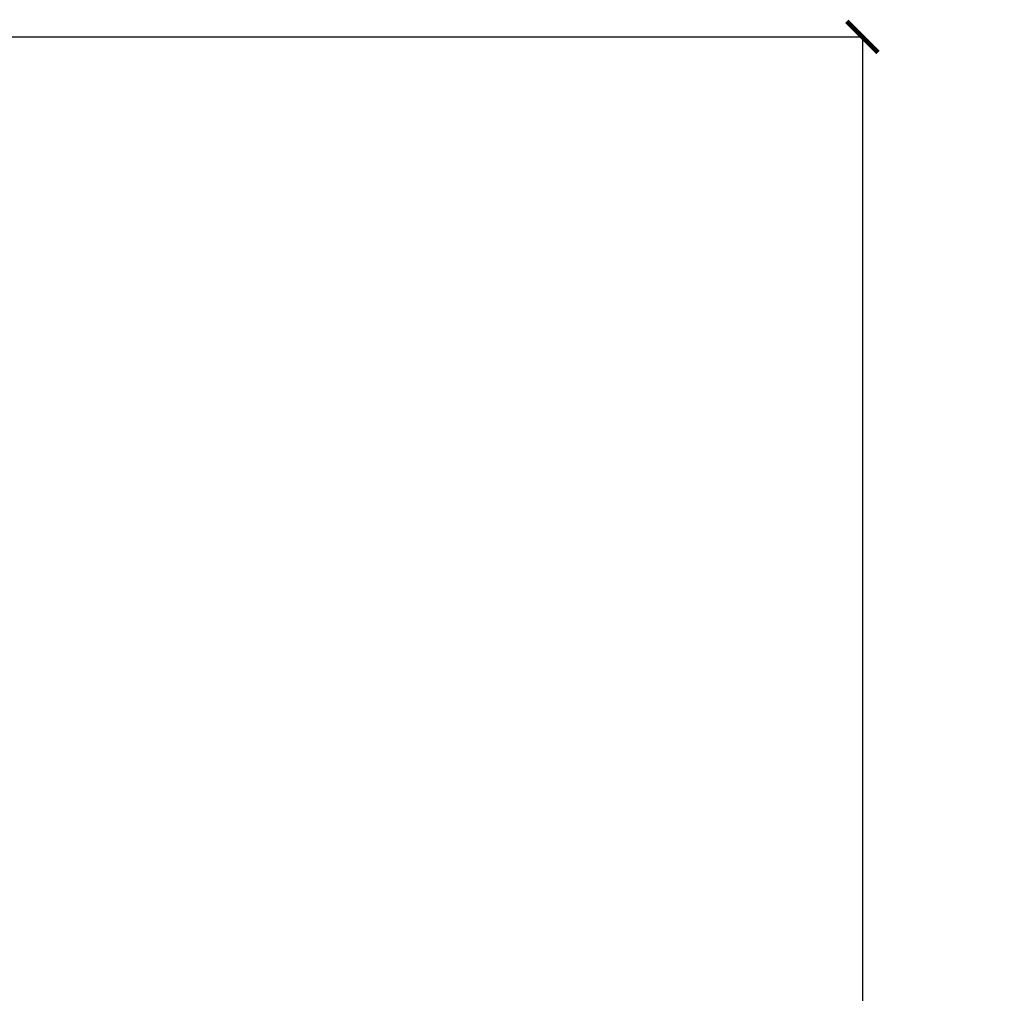
# Model space of a CAD drawing. Units: inches. Extents: x 1704 to 6393, y -157 to 1172.
# Tile 115 of 122: x 2730 to 2793, y 972 to 1034. Entities that reach past the tile are written whole.
import ezdxf

# ---------------------------------------------------------------- set-up
doc = ezdxf.new("R2010")
doc.units = ezdxf.units.IN
doc.header["$MEASUREMENT"] = 0
doc.layers.add('A-ANNO-DIMS', color=7, linetype='Continuous', lineweight=13)
doc.styles.get("Standard").update_dxf_attribs({"font": 'arial.ttf'})
doc.dimstyles.get("Standard").update_dxf_attribs({"dimtxt": 6, "dimasz": 2, "dimexe": 0.18, "dimexo": 0.0625, "dimgap": 0.09, "dimtad": 0, "dimtih": 1, "dimtoh": 1, "dimdec": 1, "dimzin": 0, "dimdsep": 46, "dimlunit": 3, "dimtxsty": 'Standard', "dimblk": 'ARCHTICK', "dimcen": 0.09, "dimadec": 0, "dimazin": 0, "dimtfac": 1, "dimtdec": 1, "dimtofl": 0, "dimtmove": 0, "dimatfit": 3, "dimfxl": 1, "dimtolj": 1, "dimtzin": 0, "dimarcsym": 0})

# ---------------------------------------------------------------- blocks, each defined once
blk = doc.blocks.new('_ArchTick')
at = {"color": 0, "linetype": 'ByBlock', "const_width": 0.15}
blk.add_lwpolyline([(-0.5, -0.5), (0.5, 0.5)], dxfattribs=at)
blk = doc.blocks.new('*D91')
at = {"layer": 'A-ANNO-DIMS', "color": 0, "lineweight": -2, "transparency": 16777216}
for p, q in [((2723.411, 1033.213), (2784.529, 1033.213)), ((2784.349, 1033.213), (2784.349, 517.868)), ((2784.349, -3.787), (2784.349, 511.557)), ((2723.411, -3.787), (2784.529, -3.787))]:
    blk.add_line(p, q, dxfattribs=at)
at = {"layer": 'Defpoints', "color": 0, "lineweight": -3, "transparency": 16777216}
for p in [(2723.349, 1033.213), (2784.349, 1033.213), (2723.349, -3.787)]:
    blk.add_point(p, dxfattribs=at)
at = {"layer": 'A-ANNO-DIMS', "color": 0, "lineweight": -2, "transparency": 16777216, "xscale": 2, "yscale": 2, "zscale": 2}
for p, rotation in [((2784.349, 1033.213), 90), ((2784.349, -3.787), 270)]:
    blk.add_blockref('_ArchTick', p, dxfattribs=dict(at, rotation=rotation))
at = {"layer": 'A-ANNO-DIMS', "color": 0, "transparency": 16777216, "insert": (2784.349, 514.713), "char_height": 6, "attachment_point": 5}
blk.add_mtext('\\A1;1037', dxfattribs=at)

msp = doc.modelspace()

# ---------------------------------------------------------------- dimensions: what is measured, and where the dimension line sits
at = {"layer": 'A-ANNO-DIMS'}
dim = msp.add_linear_dim(base=(2784.349, 1033.213), p1=(2723.349, -3.787), p2=(2723.349, 1033.213), angle=90, dimstyle='Standard', override={"dimdec": 0, "dimlfac": 1, "dimrnd": 0, "dimzin": 0, "dimdsep": 46, "dimlunit": 2}, dxfattribs=at)
dim.commit()
dim.dimension.update_dxf_attribs({"geometry": '*D91', "text_midpoint": (2784.349, 514.713)})

doc.saveas('drawing.dxf')
